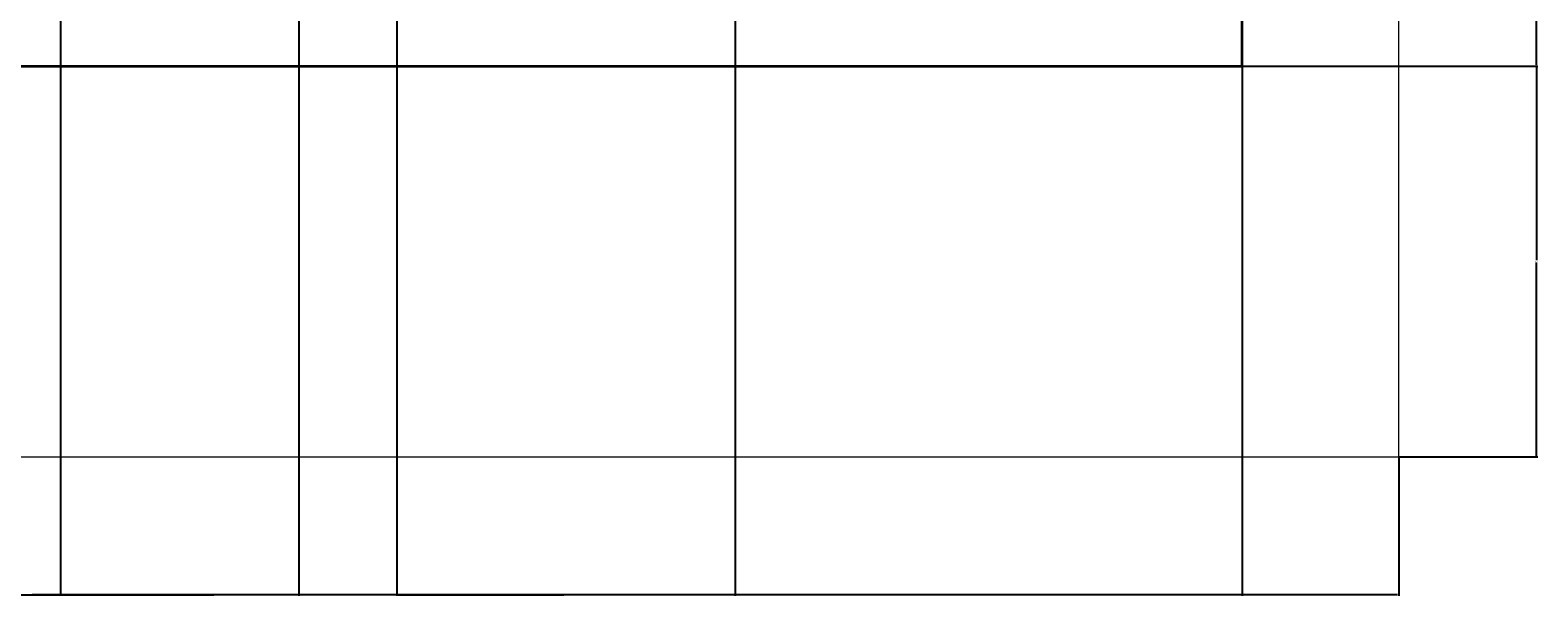
# Model space of a CAD drawing. Units: inches. Extents: x 109 to 572, y -157 to 568.
# Tile 3 of 5: x 341 to 572, y 105 to 192. Entities that reach past the tile are written whole.
import ezdxf

# ---------------------------------------------------------------- set-up
doc = ezdxf.new("R2010")
doc.units = ezdxf.units.IN
for name, color, linetype, lineweight in [('A-ANNO-DIMS', 2, 'Continuous', 18), ('A-WALL', 7, 'Continuous', 35), ('C-PROP', 8, 'Continuous', 18)]:
    doc.layers.add(name, color=color, linetype=linetype, lineweight=lineweight)
doc.styles.get("Standard").update_dxf_attribs({"font": 'arial.ttf'})
doc.dimstyles.get("Standard").update_dxf_attribs({"dimtxt": 0.18, "dimasz": 0.18, "dimexe": 0.18, "dimexo": 0.0625, "dimgap": 0.09, "dimtad": 0, "dimtih": 1, "dimtoh": 1, "dimdec": 4, "dimzin": 0, "dimdsep": 46, "dimtxsty": 'Standard', "dimcen": 0.09, "dimadec": 0, "dimazin": 0, "dimtfac": 1, "dimtdec": 4, "dimtofl": 0, "dimtmove": 0, "dimatfit": 3, "dimfxl": 1, "dimtolj": 1, "dimtzin": 0, "dimarcsym": 0})

# ---------------------------------------------------------------- blocks, each defined once
blk = doc.blocks.new('*D39')
at = {"layer": 'A-ANNO-DIMS', "color": 0, "lineweight": -2, "transparency": 16777216}
for p, q in [((130.52, 126.48), (130.52, 105.21)), ((550.52, 126.48), (550.52, 105.21)), ((130.7, 105.39), (340.23, 105.39)), ((550.34, 105.39), (340.81, 105.39))]:
    blk.add_line(p, q, dxfattribs=at)
at = {"layer": 'A-ANNO-DIMS', "color": 0, "transparency": 16777216}
for points in [[(130.7, 105.42), (130.7, 105.36), (130.52, 105.39)], [(550.34, 105.42), (550.34, 105.36), (550.52, 105.39)]]:
    blk.add_solid(points, dxfattribs=at)
at = {"layer": 'Defpoints', "color": 0, "transparency": 16777216}
for p in [(130.52, 126.54), (550.52, 126.54), (550.52, 105.39)]:
    blk.add_point(p, dxfattribs=at)
at = {"layer": 'A-ANNO-DIMS', "color": 0, "transparency": 16777216, "insert": (340.52, 105.39), "char_height": 0.18, "attachment_point": 5}
blk.add_mtext('\\A1;420', dxfattribs=at)
blk = doc.blocks.new('*D42')
at = {"layer": 'A-ANNO-DIMS', "color": 0, "lineweight": -2, "transparency": 16777216}
for p, q in [((526.58, 186.54), (571.85, 186.54)), ((571.67, 186.36), (571.67, 156.72)), ((571.67, 126.72), (571.67, 156.36)), ((550.58, 126.54), (571.85, 126.54))]:
    blk.add_line(p, q, dxfattribs=at)
at = {"layer": 'A-ANNO-DIMS', "color": 0, "transparency": 16777216}
for points in [[(571.64, 186.36), (571.7, 186.36), (571.67, 186.54)], [(571.64, 126.72), (571.7, 126.72), (571.67, 126.54)]]:
    blk.add_solid(points, dxfattribs=at)
at = {"layer": 'Defpoints', "color": 0, "transparency": 16777216}
for p in [(526.52, 186.54), (571.67, 186.54), (550.52, 126.54)]:
    blk.add_point(p, dxfattribs=at)
at = {"layer": 'A-ANNO-DIMS', "color": 0, "transparency": 16777216, "insert": (571.67, 156.54), "char_height": 0.18, "attachment_point": 5}
blk.add_mtext('\\A1;60', dxfattribs=at)
blk = doc.blocks.new('*D43')
at = {"layer": 'A-ANNO-DIMS', "color": 0, "lineweight": -2, "transparency": 16777216}
for p, q in [((211.52, 186.48), (211.52, 105.21)), ((526.52, 186.48), (526.52, 105.21)), ((211.7, 105.39), (368.73, 105.39)), ((526.34, 105.39), (369.31, 105.39))]:
    blk.add_line(p, q, dxfattribs=at)
at = {"layer": 'A-ANNO-DIMS', "color": 0, "transparency": 16777216}
for points in [[(211.7, 105.42), (211.7, 105.36), (211.52, 105.39)], [(526.34, 105.42), (526.34, 105.36), (526.52, 105.39)]]:
    blk.add_solid(points, dxfattribs=at)
at = {"layer": 'Defpoints', "color": 0, "transparency": 16777216}
for p in [(211.52, 186.54), (526.52, 186.54), (526.52, 105.39)]:
    blk.add_point(p, dxfattribs=at)
at = {"layer": 'A-ANNO-DIMS', "color": 0, "transparency": 16777216, "insert": (369.02, 105.39), "char_height": 0.18, "attachment_point": 5}
blk.add_mtext('\\A1;315', dxfattribs=at)
blk = doc.blocks.new('*D44')
at = {"layer": 'A-ANNO-DIMS', "color": 0, "lineweight": -2, "transparency": 16777216}
for p, q in [((526.58, 522.54), (571.85, 522.54)), ((571.67, 522.36), (571.67, 354.72)), ((571.67, 186.72), (571.67, 354.36)), ((526.58, 186.54), (571.85, 186.54))]:
    blk.add_line(p, q, dxfattribs=at)
at = {"layer": 'A-ANNO-DIMS', "color": 0, "transparency": 16777216}
for points in [[(571.64, 522.36), (571.7, 522.36), (571.67, 522.54)], [(571.64, 186.72), (571.7, 186.72), (571.67, 186.54)]]:
    blk.add_solid(points, dxfattribs=at)
at = {"layer": 'Defpoints', "color": 0, "transparency": 16777216}
for p in [(526.52, 522.54), (571.67, 522.54), (526.52, 186.54)]:
    blk.add_point(p, dxfattribs=at)
at = {"layer": 'A-ANNO-DIMS', "color": 0, "transparency": 16777216, "insert": (571.67, 354.54), "char_height": 0.18, "attachment_point": 5}
blk.add_mtext('\\A1;336', dxfattribs=at)
blk = doc.blocks.new('*D61')
at = {"layer": 'A-ANNO-DIMS', "color": 0, "lineweight": -2, "transparency": 16777216}
for p, q in [((396.8, 428.71), (396.8, 105.21)), ((448.7, 428.71), (448.7, 105.21)), ((396.98, 105.39), (422.43, 105.39)), ((448.52, 105.39), (423.08, 105.39))]:
    blk.add_line(p, q, dxfattribs=at)
at = {"layer": 'A-ANNO-DIMS', "color": 0, "transparency": 16777216}
for points in [[(396.98, 105.42), (396.98, 105.36), (396.8, 105.39)], [(448.52, 105.42), (448.52, 105.36), (448.7, 105.39)]]:
    blk.add_solid(points, dxfattribs=at)
at = {"layer": 'Defpoints', "color": 0, "transparency": 16777216}
for p in [(396.8, 428.77), (448.7, 428.77), (448.7, 105.39)]:
    blk.add_point(p, dxfattribs=at)
at = {"layer": 'A-ANNO-DIMS', "color": 0, "transparency": 16777216, "insert": (422.75, 105.39), "char_height": 0.18, "attachment_point": 5}
blk.add_mtext('\\A1;51.9', dxfattribs=at)
blk = doc.blocks.new('*D71')
at = {"layer": 'A-ANNO-DIMS', "color": 0, "lineweight": -2, "transparency": 16777216}
for p, q in [((345.17, 436.98), (345.17, 105.21)), ((381.74, 436.98), (381.74, 105.21)), ((345.35, 105.39), (363.06, 105.39)), ((381.56, 105.39), (363.85, 105.39))]:
    blk.add_line(p, q, dxfattribs=at)
at = {"layer": 'A-ANNO-DIMS', "color": 0, "transparency": 16777216}
for points in [[(345.35, 105.42), (345.35, 105.36), (345.17, 105.39)], [(381.56, 105.42), (381.56, 105.36), (381.74, 105.39)]]:
    blk.add_solid(points, dxfattribs=at)
at = {"layer": 'Defpoints', "color": 0, "transparency": 16777216}
for p in [(345.17, 437.04), (381.74, 437.04), (381.74, 105.39)]:
    blk.add_point(p, dxfattribs=at)
at = {"layer": 'A-ANNO-DIMS', "color": 0, "transparency": 16777216, "insert": (363.46, 105.39), "char_height": 0.18, "attachment_point": 5}
blk.add_mtext('\\A1;36.57', dxfattribs=at)

msp = doc.modelspace()

# ---------------------------------------------------------------- linework, layer by layer
at = {"layer": 'A-WALL'}
for p, q in [((526.5195, 186.5398), (526.5195, 522.5398)), ((211.5195, 186.5398), (526.5195, 186.5398))]:
    msp.add_line(p, q, dxfattribs=at)
at = {"layer": 'C-PROP'}
for p, q in [((550.5195, 126.5398), (550.5195, 546.5398)), ((130.5195, 126.5398), (550.5195, 126.5398))]:
    msp.add_line(p, q, dxfattribs=at)

# ---------------------------------------------------------------- dimensions: what is measured, and where the dimension line sits
at = {"layer": 'A-ANNO-DIMS'}
for base, p1, p2, picture, middle in [((571.6695, 522.5398), (526.5195, 186.5398), (526.5195, 522.5398), '*D44', (571.6695, 354.5398)), ((571.6695, 186.5398), (550.5195, 126.5398), (526.5195, 186.5398), '*D42', (571.6695, 156.5398))]:
    dim = msp.add_linear_dim(base=base, p1=p1, p2=p2, angle=90, dimstyle='Standard', override={"dimdec": 0, "dimlfac": 1, "dimrnd": 0, "dimzin": 0, "dimdsep": 46, "dimlunit": 2}, dxfattribs=at)
    dim.commit()
    dim.dimension.update_dxf_attribs({"geometry": picture, "text_midpoint": middle})
for base, p1, p2, override, picture, middle in [((381.7416, 105.3898), (345.1719, 437.0398), (381.7416, 437.0398), {"dimdec": 2, "dimlfac": 1, "dimrnd": 0, "dimzin": 0, "dimdsep": 46, "dimlunit": 2}, '*D71', (363.4567, 105.3898)), ((448.7025, 105.3898), (396.8044, 428.7734), (448.7025, 428.7734), {"dimdec": 1, "dimlfac": 1, "dimrnd": 0, "dimzin": 0, "dimdsep": 46, "dimlunit": 2}, '*D61', (422.7534, 105.3898)), ((526.5195, 105.3898), (211.5195, 186.5398), (526.5195, 186.5398), {"dimdec": 0, "dimlfac": 1, "dimrnd": 0, "dimzin": 0, "dimdsep": 46, "dimlunit": 2}, '*D43', (369.0195, 105.3898)), ((550.5195, 105.3898), (130.5195, 126.5398), (550.5195, 126.5398), {"dimdec": 0, "dimlfac": 1, "dimrnd": 0, "dimzin": 0, "dimdsep": 46, "dimlunit": 2}, '*D39', (340.5195, 105.3898))]:
    dim = msp.add_linear_dim(base=base, p1=p1, p2=p2, dimstyle='Standard', override=override, dxfattribs=at)
    dim.commit()
    dim.dimension.update_dxf_attribs({"geometry": picture, "text_midpoint": middle})

doc.saveas('drawing.dxf')
